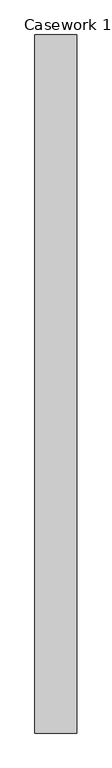
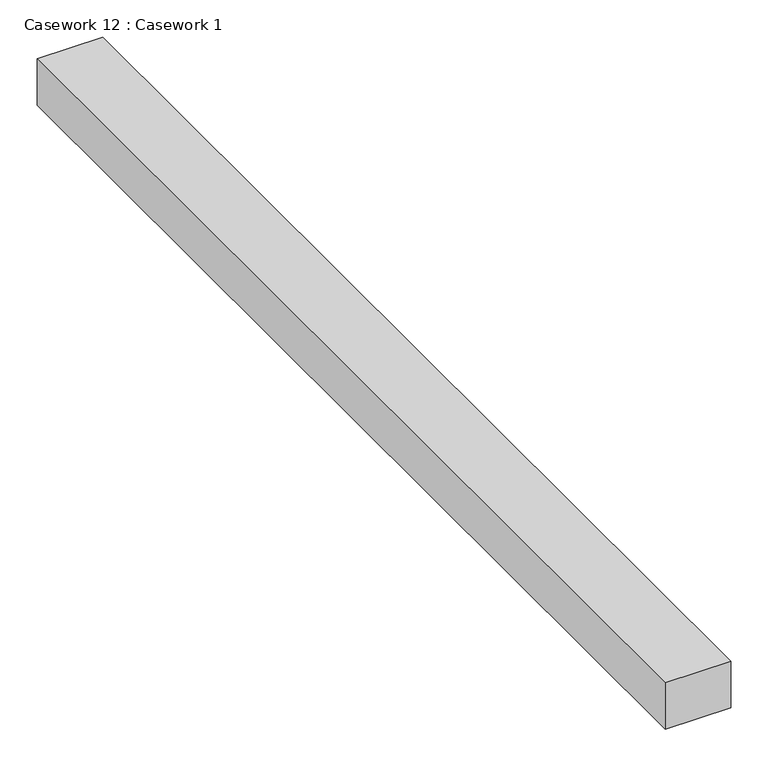
"""IFC4 building model written with IfcOpenShell, lengths in millimetres: furniture geometry, Casework 12 : Casework 1."""

from ifc_helpers import new_model, si_unit, frame, origin, place, context, project, spatial, polyline, outline, extrude, source, transform, mapped, element, save


def casework_12_casework_1_dcbad799(model_context):
    return source(origin(), model_context, "Body", "SweptSolid", [
        extrude(outline(polyline([(6309.7559589, 14787.9496924), (6309.7559589, 13098.8496924), (6208.1559589, 13098.8496924), (6208.1559589, 14787.9496924), (6309.7559589, 14787.9496924)])), frame((0.0, 0.0, 3581.4), z_axis=(0.0, 0.0, 1.0), x_axis=(1.0, 0.0, 0.0)), (0.0, 0.0, 1.0), 76.2),
    ])


if __name__ == "__main__":
    model = new_model("IFC4")
    model_context = context("Model", 3, world=origin())
    ifc_project = project(units=[si_unit("LENGTHUNIT", "METRE", prefix="MILLI")], contexts=[model_context])
    site = spatial("IfcSite", under=ifc_project)
    building = spatial("IfcBuilding", under=site)
    placement = place(None, origin())
    casework_12_casework_1_shape = casework_12_casework_1_dcbad799(model_context)
    element("IfcFurniture", 1, ObjectType="Casework 12 : Casework 1", at=placement, inside=building, context=model_context, shape_type="MappedRepresentation", body=[
        mapped(casework_12_casework_1_shape, transform((0.0, 0.0, 0.0), x_axis=(1.0, 0.0, 0.0), y_axis=(0.0, 1.0, 0.0), z_axis=(0.0, 0.0, 1.0))),
    ])
    save(model, "model.ifc")

# Revit data of these elements
# Element 1 (IfcFurniture, "Casework 12 : Casework 1")
#   Materials on its faces: "Clad - White"
# Materials
#   "Clad - White": class "Wood", colour RGB 242 242 238, transparency 0, Cost = 0
